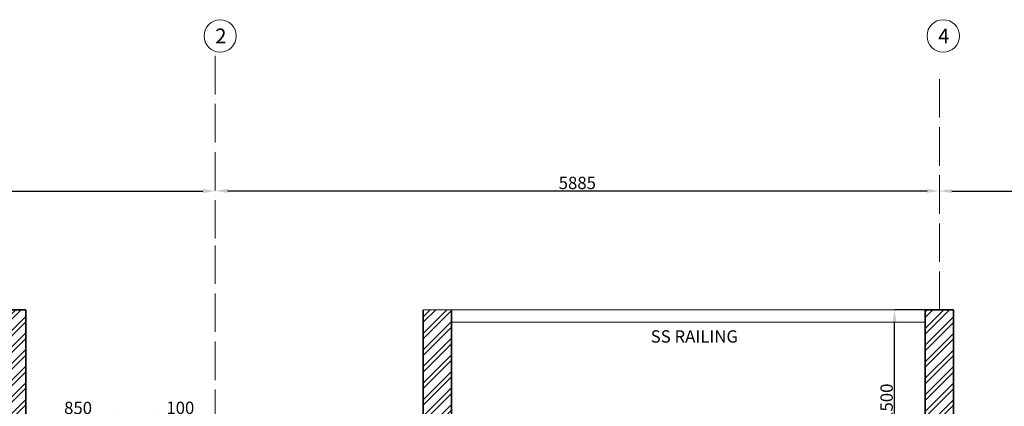
# Model space of a CAD drawing. Units: millimetres. Extents: x -3326 to 29338, y -16792 to 6002.
# Tile 11 of 21: x 3793 to 11795, y 2813 to 5952. Entities that reach past the tile are written whole.
import ezdxf

# ---------------------------------------------------------------- set-up
doc = ezdxf.new("R2010")
doc.units = ezdxf.units.MM
doc.header["$PDMODE"] = 35
doc.header["$PDSIZE"] = 5
doc.linetypes.add('ACAD_ISO04W100', pattern=[30, 24, -3, 0, -3])
for name, color, linetype, lineweight in [('A-ANNO-DIMS', 2, 'Continuous', 13), ('A-FLOR-RAIL', 8, 'Continuous', 20), ('A-GRID', 8, 'ACAD_ISO04W100', 13), ('A-GRID-IDEN', 7, 'Continuous', 18), ('A-WALL', 7, 'Continuous', 35), ('A-WALL-PATT', 252, 'Continuous', 13), ('txt', 7, 'Continuous', 18)]:
    doc.layers.add(name, color=color, linetype=linetype, lineweight=lineweight)
doc.styles.get("Standard").update_dxf_attribs({"font": 'arial.ttf'})
doc.dimstyles.new('ISO-25', dxfattribs={"dimtxt": 100, "dimasz": 100, "dimexe": 1.25, "dimexo": 0.625, "dimtad": 1, "dimtxsty": 'Standard', "dimcen": 2.5, "dimadec": 0, "dimazin": 0, "dimtfac": 1, "dimtmove": 0, "dimatfit": 3, "dimfxl": 1, "dimarcsym": 0})
pattern_1 = [(45, (-10476.65, 1e-12), (-67.35192, 67.35192), []), (45, (-10431.74, 1e-12), (-67.35192, 67.35192), [])]

# ---------------------------------------------------------------- blocks, each defined once
blk = doc.blocks.new('*D127')
at = {"layer": 'A-ANNO-DIMS', "color": 0, "lineweight": -2, "transparency": 16777216}
for p, q in [((11151.7, 3596), (10901.5, 3596)), ((10902.7, 2196), (10902.7, 3496)), ((11151.7, 2096), (10901.5, 2096))]:
    blk.add_line(p, q, dxfattribs=at)
at = {"layer": 'A-ANNO-DIMS', "color": 0, "transparency": 16777216}
for points in [[(10886.1, 3496), (10919.4, 3496), (10902.7, 3596)], [(10886.1, 2196), (10919.4, 2196), (10902.7, 2096)]]:
    blk.add_solid(points, dxfattribs=at)
at = {"layer": 'Defpoints', "color": 0, "transparency": 16777216}
for p in [(10902.7, 3596), (11152.3, 3596), (11152.3, 2096)]:
    blk.add_point(p, dxfattribs=at)
at = {"layer": 'A-ANNO-DIMS', "color": 0, "transparency": 16777216, "insert": (10851.1, 2846), "char_height": 100, "attachment_point": 5, "rotation": 90}
blk.add_mtext('1500', dxfattribs=at)
blk = doc.blocks.new('*D146')
at = {"layer": 'A-ANNO-DIMS', "color": 0, "lineweight": -2, "transparency": 16777216}
for p, q in [((4592.3, 2736.2), (4492.3, 2736.2)), ((4692.3, 2496.7), (4692.3, 2737.4)), ((4692.3, 2736.2), (4792.3, 2736.2)), ((4792.3, 2496.7), (4792.3, 2737.4)), ((4892.3, 2736.2), (5204.7, 2736.2))]:
    blk.add_line(p, q, dxfattribs=at)
at = {"layer": 'A-ANNO-DIMS', "color": 0, "transparency": 16777216}
for points in [[(4592.3, 2752.9), (4592.3, 2719.5), (4692.3, 2736.2)], [(4892.3, 2752.9), (4892.3, 2719.5), (4792.3, 2736.2)]]:
    blk.add_solid(points, dxfattribs=at)
at = {"layer": 'Defpoints', "color": 0, "transparency": 16777216}
for p in [(4792.3, 2736.2), (4692.3, 2496), (4792.3, 2496)]:
    blk.add_point(p, dxfattribs=at)
at = {"layer": 'A-ANNO-DIMS', "color": 0, "transparency": 16777216, "insert": (5098.5, 2787.9), "char_height": 100, "attachment_point": 5}
blk.add_mtext('100', dxfattribs=at)
blk = doc.blocks.new('*D149')
at = {"layer": 'A-ANNO-DIMS', "color": 0, "lineweight": -2, "transparency": 16777216}
for p, q in [((3842.3, 2617.7), (3842.3, 2736.3)), ((4592.3, 2735), (3942.3, 2735)), ((4692.3, 2617.7), (4692.3, 2736.3))]:
    blk.add_line(p, q, dxfattribs=at)
at = {"layer": 'A-ANNO-DIMS', "color": 0, "transparency": 16777216}
for points in [[(3942.3, 2751.7), (3942.3, 2718.4), (3842.3, 2735)], [(4592.3, 2751.7), (4592.3, 2718.4), (4692.3, 2735)]]:
    blk.add_solid(points, dxfattribs=at)
at = {"layer": 'Defpoints', "color": 0, "transparency": 16777216}
for p in [(3842.3, 2735), (3842.3, 2617.1), (4692.3, 2617.1)]:
    blk.add_point(p, dxfattribs=at)
at = {"layer": 'A-ANNO-DIMS', "color": 0, "transparency": 16777216, "insert": (4267.3, 2786.7), "char_height": 100, "attachment_point": 5}
blk.add_mtext('850', dxfattribs=at)
blk = doc.blocks.new('*D152')
at = {"layer": 'A-ANNO-DIMS', "color": 0, "lineweight": -2, "transparency": 16777216}
for p, q in [((-506.2, 4561.1), (-506.2, 4561.8)), ((5382.3, 4561.1), (5382.3, 4561.8)), ((-406.2, 4560.5), (5282.3, 4560.5))]:
    blk.add_line(p, q, dxfattribs=at)
at = {"layer": 'A-ANNO-DIMS', "color": 0, "transparency": 16777216}
for points in [[(-406.2, 4577.2), (-406.2, 4543.8), (-506.2, 4560.5)], [(5282.3, 4577.2), (5282.3, 4543.8), (5382.3, 4560.5)]]:
    blk.add_solid(points, dxfattribs=at)
at = {"layer": 'Defpoints', "color": 0, "transparency": 16777216}
for p in [(-506.2, 4560.5), (5382.3, 4560.5), (5382.3, 4560.5)]:
    blk.add_point(p, dxfattribs=at)
at = {"layer": 'A-ANNO-DIMS', "color": 0, "transparency": 16777216, "insert": (2438, 4621.2), "char_height": 100, "attachment_point": 5}
blk.add_mtext('5888,52', dxfattribs=at)
blk = doc.blocks.new('*D153')
at = {"layer": 'A-ANNO-DIMS', "color": 0, "lineweight": -2, "transparency": 16777216}
for p, q in [((5382.3, 4562.4), (5382.3, 4563)), ((5482.3, 4561.8), (11167.3, 4561.8)), ((11267.3, 4562.4), (11267.3, 4563))]:
    blk.add_line(p, q, dxfattribs=at)
at = {"layer": 'A-ANNO-DIMS', "color": 0, "transparency": 16777216}
for points in [[(5482.3, 4578.4), (5482.3, 4545.1), (5382.3, 4561.8)], [(11167.3, 4578.4), (11167.3, 4545.1), (11267.3, 4561.8)]]:
    blk.add_solid(points, dxfattribs=at)
at = {"layer": 'Defpoints', "color": 0, "transparency": 16777216}
for p in [(5382.3, 4561.8), (11267.3, 4561.8), (11267.3, 4561.8)]:
    blk.add_point(p, dxfattribs=at)
at = {"layer": 'A-ANNO-DIMS', "color": 0, "transparency": 16777216, "insert": (8324.8, 4613.4), "char_height": 100, "attachment_point": 5}
blk.add_mtext('5885', dxfattribs=at)
blk = doc.blocks.new('*D154')
at = {"layer": 'A-ANNO-DIMS', "color": 0, "lineweight": -2, "transparency": 16777216}
for p, q in [((11267.3, 4562.4), (11267.3, 4559.3)), ((17397.3, 4561.1), (17397.3, 4561.8)), ((11367.3, 4560.5), (17297.3, 4560.5))]:
    blk.add_line(p, q, dxfattribs=at)
at = {"layer": 'A-ANNO-DIMS', "color": 0, "transparency": 16777216}
for points in [[(11367.3, 4577.2), (11367.3, 4543.8), (11267.3, 4560.5)], [(17297.3, 4577.2), (17297.3, 4543.8), (17397.3, 4560.5)]]:
    blk.add_solid(points, dxfattribs=at)
at = {"layer": 'Defpoints', "color": 0, "transparency": 16777216}
for p in [(11267.3, 4563), (17397.3, 4560.5), (17397.3, 4560.5)]:
    blk.add_point(p, dxfattribs=at)
at = {"layer": 'A-ANNO-DIMS', "color": 0, "transparency": 16777216, "insert": (14332.3, 4612.2), "char_height": 100, "attachment_point": 5}
blk.add_mtext('6130', dxfattribs=at)

msp = doc.modelspace()

# ---------------------------------------------------------------- hatches: boundary and pattern name
at = {"layer": 'A-WALL-PATT'}
h = msp.add_hatch(dxfattribs=at)
h.set_pattern_fill('ANSI32', color=256, scale=10)
h.set_pattern_definition(pattern_1)
h.paths.add_polyline_path([(2842.301, -2383.952), (-215.519, -2383.952), (-215.519, -2483.952), (1282.301, -2483.952), (1282.301, -2683.952), (1413.549, -2683.952), (1413.549, -2680.395), (1493.875, -2680.395), (1512.301, -2683.952), (1512.301, -2483.952), (2842.301, -2483.952)])
h.paths.add_polyline_path([(1512.301, -3583.952), (1493.875, -3583.952), (1493.875, -3584.058), (1413.549, -3584.058), (1282.301, -3583.952), (1282.301, -4183.952), (1512.301, -4183.952)])
h.paths.add_polyline_path([(5172.301, -1733.952), (3842.301, -1733.952), (3742.301, -1733.952), (3742.301, -1833.952), (3742.301, -2389.299), (3746.327, -2389.299), (3746.327, -2469.299), (3742.301, -2469.299), (3742.301, -2483.952), (3842.301, -2483.952), (3842.301, -1833.952), (5172.301, -1833.952)])
h.paths.add_polyline_path([(5572.301, 1346.048), (5342.301, 1346.048), (5342.301, -733.952), (4642.301, -733.952), (4642.301, -833.952), (5342.301, -833.952), (5342.301, -1733.952), (5572.301, -1733.952), (5572.301, -1033.952), (6402.301, -1033.952), (6402.301, -933.952), (5572.301, -933.952)])
h.paths.add_polyline_path([(4092.301, 2096.048), (3842.301, 2096.048), (3842.301, 3596.048), (3612.301, 3596.048), (3612.301, 2096.048), (3282.301, 2096.048), (3282.301, 1866.048), (3612.301, 1866.048), (3742.301, 1866.048), (3742.301, -1733.952), (3842.301, -1733.952), (3842.301, -815.784), (3839.26, -815.784), (3839.26, -735.784), (3842.301, 1866.048), (4092.301, 1866.048)])
h.paths.add_polyline_path([(7302.301, 3596.048), (7072.301, 3596.048), (7072.301, 2096.048), (6672.301, 2096.048), (6672.301, 1866.048), (7202.301, 1866.048), (7202.301, -943.25), (7207.296, -943.25), (7207.296, -1023.25), (7202.301, -1033.952), (7217.026, -1033.952), (7217.026, -1030.415), (7302.301, -1030.415), (7302.301, 1866.048), (7302.301, 1946.048)])
h.paths.add_polyline_path([(6072.301, 2096.048), (5572.301, 2096.048), (5572.301, 1866.048), (6072.301, 1866.048)])
h.paths.add_polyline_path([(5172.301, 2096.048), (4692.301, 2096.048), (4692.301, 1866.048), (5172.301, 1866.048)])
h.paths.add_polyline_path([(4792.301, 2496.048), (4692.301, 2496.048), (4692.301, 2096.048), (4792.301, 2096.048)])
h.paths.add_polyline_path([(6072.301, 2496.048), (5972.301, 2496.048), (5972.301, 2096.048), (6072.301, 2096.048)])
h.paths.add_polyline_path([(1482.301, 2096.048), (1132.301, 2096.048), (1132.301, 1866.048), (1482.301, 1866.048)])
h.paths.add_polyline_path([(232.301, 2096.048), (-217.699, 2096.048), (-217.699, 1866.048), (232.301, 1866.048), (232.301, 1876.048), (226.22, 1876.048), (226.22, 1956.048)])
h.paths.add_polyline_path([(-387.699, 3596.048), (-394.734, 3596.048), (-617.699, 3596.048), (-617.699, 2096.048), (-387.699, 2096.048)])
h.paths.add_polyline_path([(-387.699, 1596.048), (-617.699, 1596.048), (-617.699, 336.048), (-617.699, -1883.952), (-215.519, -1883.952), (-215.519, -1783.952), (-387.699, -1783.952)])
h = msp.add_hatch(dxfattribs=at)
h.set_pattern_fill('ANSI32', color=256, scale=10)
h.set_pattern_definition(pattern_1)
h.paths.add_polyline_path([(12212.301, -1983.952), (11640.861, -1983.952), (11640.861, -2213.952), (12212.301, -2213.952)])
h.paths.add_polyline_path([(14712.301, -1983.952), (14012.301, -1983.952), (14012.301, -2213.952), (14712.301, -2213.952)])
h.paths.add_polyline_path([(17012.301, -1983.952), (16512.301, -1983.952), (16512.301, -2213.952), (17012.301, -2213.952)])
h.paths.add_polyline_path([(11382.301, -2383.952), (11040.861, -2383.952), (7302.301, -2383.952), (7302.301, -1935.766), (7217.026, -1935.766), (7202.301, -1933.952), (7202.301, -2483.952), (7302.301, -2483.952), (11152.301, -2483.952), (11152.301, -2833.952), (11283.549, -2833.952), (11283.549, -2830.395), (11363.875, -2830.395), (11382.301, -2833.952)])
h.paths.add_polyline_path([(11382.301, -3733.952), (11363.875, -3733.952), (11363.875, -3734.058), (11283.549, -3734.058), (11152.301, -3733.952), (11152.301, -6450.401), (11382.301, -6450.401)])
h.paths.add_polyline_path([(13462.301, -6450.401), (12606.738, -6450.401), (11382.301, -6450.401), (11382.301, -6680.401), (12606.738, -6680.401), (13462.301, -6680.401)])
h.paths.add_polyline_path([(11382.301, -7050.401), (11152.301, -7050.401), (11152.301, -8810.401), (11382.301, -8810.401)])
h.paths.add_polyline_path([(13462.301, -8980.401), (11751.174, -8980.401), (11751.174, -9210.401), (13462.301, -9210.401)])
h.paths.add_polyline_path([(13962.301, -6850.401), (13732.301, -6850.401), (13732.301, -7350.401), (13962.301, -7350.401)])
h.paths.add_polyline_path([(13962.301, -8309.482), (13732.301, -8309.482), (13732.301, -8809.482), (13962.301, -8809.482)])
h.paths.add_polyline_path([(15712.301, -12533.952), (12902.301, -12533.952), (12902.301, -12763.952), (15712.301, -12763.952)])
h.paths.add_polyline_path([(11508.301, -9211.585), (11382.301, -9211.585), (11152.301, -9211.585), (11152.301, -11033.952), (10952.301, -11033.952), (10952.301, -11263.952), (11152.301, -11263.952), (11152.301, -12361.585), (11508.301, -12361.585)])
h.paths.add_polyline_path([(12002.301, -12533.952), (11902.301, -12533.952), (11902.301, -12761.585), (11152.301, -12761.585), (11152.301, -12763.952), (11902.301, -12763.952), (12002.301, -12763.952)])
h.paths.add_polyline_path([(17112.301, -12533.952), (16912.301, -12533.952), (16912.301, -12763.952), (17112.301, -12763.952)])
h.paths.add_polyline_path([(11382.301, 3596.048), (11152.301, 3596.048), (11152.301, 2096.048), (11382.301, 2096.048)])
h.paths.add_polyline_path([(11382.301, 1496.048), (11152.301, 1496.048), (11152.301, -1983.952), (11382.301, -1983.952)])

# ---------------------------------------------------------------- linework, layer by layer
at = {"layer": 'A-FLOR-RAIL'}
for p, q in [((7302.301, 3596.048), (7072.301, 3596.048)), ((11152.301, 3596.048), (7302.301, 3596.048)), ((11152.301, 3496.048), (7302.301, 3496.048))]:
    msp.add_line(p, q, dxfattribs=at)
at = {"layer": 'A-GRID', "ltscale": 13}
for p, q in [((5382.301, 4174.981), (5382.301, 5719.227)), ((11267.301, 3596.048), (11267.301, 5524.981)), ((5382.301, 2246.048), (5382.301, 4174.981))]:
    msp.add_line(p, q, dxfattribs=at)
at = {"layer": 'A-GRID-IDEN'}
for centre, radius in [((5422.042, 5819.473), 130.903), ((11298.628, 5819.718), 131.819)]:
    msp.add_circle(centre, radius, dxfattribs=at)
at = {"layer": 'A-WALL'}
for p, q in [((3842.301, 3596.048), (3612.301, 3596.048)), ((3842.301, 3596.048), (3842.301, 2096.048)), ((7072.301, 3596.048), (7072.301, 2096.048)), ((7302.301, 3596.048), (7302.301, 1866.048)), ((11152.301, 3596.048), (11152.301, 2096.048)), ((11382.301, 3596.048), (11152.301, 3596.048)), ((11382.301, 3596.048), (11382.301, -1983.952))]:
    msp.add_line(p, q, dxfattribs=at)

# ---------------------------------------------------------------- texts
at = {"layer": 'A-GRID-IDEN', "char_height": 120, "attachment_point": 1}
for s, insert in [('2', (5382.301, 5879.718)), ('4', (11257.127, 5879.718))]:
    msp.add_mtext_dynamic_manual_height_columns(s, width=463.74815, gutter_width=12.5, heights=[0], dxfattribs=dict(at, insert=insert))
at = {"layer": 'txt', "insert": (8921.205, 3429.79), "char_height": 100, "attachment_point": 1}
msp.add_mtext_dynamic_manual_height_columns('SS RAILING', width=1168.90663, gutter_width=12.5, heights=[0], dxfattribs=at)

# ---------------------------------------------------------------- dimensions: what is measured, and where the dimension line sits
at = {"layer": 'A-ANNO-DIMS'}
for base, p1, p2, picture, middle in [((5382.301, 4560.514), (-506.217, 4560.514), (5382.301, 4560.514), '*D152', (2438.042, 4621.235)), ((11267.301, 4561.764), (5382.301, 4561.764), (11267.301, 4561.764), '*D153', (8324.801, 4613.447)), ((17397.301, 4560.514), (11267.301, 4563.014), (17397.301, 4560.514), '*D154', (14332.301, 4612.231)), ((3842.301, 2735.037), (4692.301, 2617.058), (3842.301, 2617.058), '*D149', (4267.301, 2786.72)), ((4792.301, 2736.193), (4692.301, 2496.048), (4792.301, 2496.048), '*D146', (5098.519, 2787.875))]:
    dim = msp.add_linear_dim(base=base, p1=p1, p2=p2, dimstyle='ISO-25', override={"dimclrd": 0, "dimclre": 0, "dimclrt": 0}, dxfattribs=at)
    dim.commit()
    dim.dimension.update_dxf_attribs({"geometry": picture, "text_midpoint": middle})
dim = msp.add_linear_dim(base=(10902.735, 3596.048), p1=(11152.301, 2096.048), p2=(11152.301, 3596.048), angle=90, dimstyle='ISO-25', override={"dimclrd": 0, "dimclre": 0, "dimclrt": 0}, dxfattribs=at)
dim.commit()
dim.dimension.update_dxf_attribs({"geometry": '*D127', "text_midpoint": (10851.053, 2846.048)})

doc.saveas('drawing.dxf')
